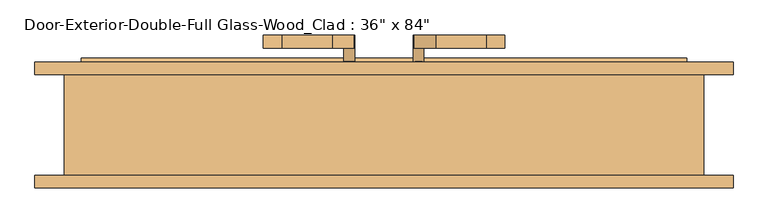
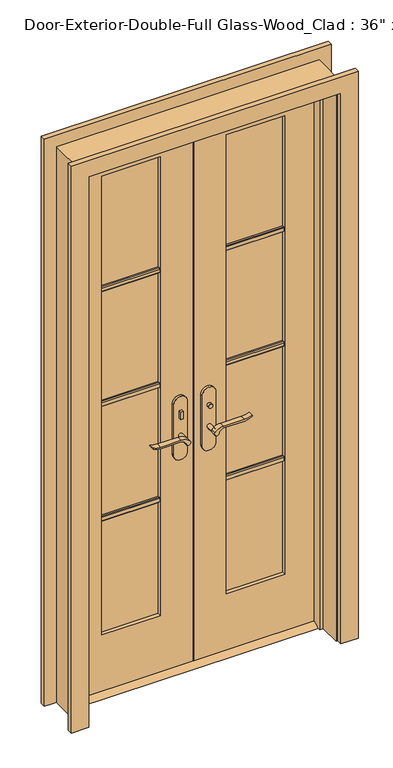
"""IFC4 building model written with IfcOpenShell, lengths in millimetres: door geometry."""

from ifc_helpers import new_model, si_unit, point, frame, frame_2d, origin, place, context, project, spatial, polyline, circle_curve, trimmed, segment, composite_curve, outline, extrude, faceted_brep, source, transform, mapped, element, save


def door_665efd91(model_context):
    return source(origin(), model_context, "Body", "SolidModel", [
        extrude(outline(polyline([(38.1, 12.7), (73.025, 12.7), (98.425, 0.0), (12.7, 0.0), (38.1, 12.7)])), frame((-457.2, 0.0, 0.0), z_axis=(1.0, 0.0, 0.0), x_axis=(0.0, 1.0, 0.0)), (0.0, 0.0, 1.0), 914.4),
        extrude(outline(polyline([(-47.4019111, 18.1), (-57.4019111, 18.1), (-57.4019111, 28.1), (-47.4019111, 28.1), (-47.4019111, 18.1)])), frame((0.0, 0.0, 981.9), z_axis=(0.0, 0.0, 1.0), x_axis=(1.0, 0.0, 0.0)), (0.0, 0.0, 1.0), 30.0),
        extrude(outline(composite_curve([segment(trimmed(circle_curve(frame_2d((996.9, -52.4019111)), 8.0), [point((996.9, -60.4019111))], [point((996.9, -44.4019111))], False, "CARTESIAN"), True, "CONTINUOUS"), segment(trimmed(circle_curve(frame_2d((996.9, -52.4019111)), 8.0), [point((996.9, -44.4019111))], [point((996.9, -60.4019111))], False, "CARTESIAN"), True, "CONTINUOUS")], self_intersect=False)), frame((0.0, 83.025, 0.0), z_axis=(0.0, 1.0, 0.0), x_axis=(0.0, 0.0, 1.0)), (0.0, 0.0, 1.0), 10.0),
        extrude(outline(composite_curve([segment(trimmed(circle_curve(frame_2d((897.1555521, -76.0694241)), 37.2832219), [point((919.0523287, -45.8937749))], [point((934.4, -77.7693445))], False, "CARTESIAN"), True, "CONTINUOUS"), segment(polyline([(934.4, -77.7693445), (934.4, -154.045502)]), True, "CONTINUOUS"), segment(trimmed(circle_curve(frame_2d((1017.6850638, -153.9791202)), 83.2850902), [point((934.4, -154.045502))], [point((939.4, -182.4019111))], True, "CARTESIAN"), True, "CONTINUOUS"), segment(polyline([(939.4, -182.4019111), (936.6135558, -182.4019111)]), True, "CONTINUOUS"), segment(trimmed(circle_curve(frame_2d((986.6709207, -150.4622499)), 59.3791355), [point((936.6135558, -182.4019111))], [point((927.4, -154.045502))], False, "CARTESIAN"), True, "CONTINUOUS"), segment(polyline([(927.4, -154.045502), (927.4, -77.7881013)]), True, "CONTINUOUS"), segment(trimmed(circle_curve(frame_2d((909.2738613, -77.7881013)), 18.1261387), [point((927.4, -77.7881013))], [point((914.4, -60.4019111))], True, "CARTESIAN"), True, "CONTINUOUS"), segment(trimmed(circle_curve(frame_2d((914.4, -52.4019111)), 8.0), [point((914.4, -60.4019111))], [point((919.0523287, -45.8937749))], False, "CARTESIAN"), True, "CONTINUOUS")], self_intersect=False)), frame((0.0, -21.9, 0.0), z_axis=(0.0, 1.0, 0.0), x_axis=(0.0, 0.0, 1.0)), (0.0, 0.0, 1.0), 20.0),
        extrude(outline(composite_curve([segment(trimmed(circle_curve(frame_2d((914.4, -52.4019111)), 8.0), [point((914.3999903, -60.4019111))], [point((919.0523287, -45.8937749))], False, "CARTESIAN"), True, "CONTINUOUS"), segment(trimmed(circle_curve(frame_2d((897.1555521, -76.0694241)), 37.2832219), [point((919.0523287, -45.8937749))], [point((934.4, -77.7693445))], False, "CARTESIAN"), True, "CONTINUOUS"), segment(polyline([(934.4, -77.7693445), (934.4, -154.045502)]), True, "CONTINUOUS"), segment(trimmed(circle_curve(frame_2d((1017.6850638, -153.9791202)), 83.2850902), [point((934.4, -154.045502))], [point((939.4, -182.4019111))], True, "CARTESIAN"), True, "CONTINUOUS"), segment(polyline([(939.4, -182.4019111), (936.6135558, -182.4019111)]), True, "CONTINUOUS"), segment(trimmed(circle_curve(frame_2d((986.6709207, -150.4622499)), 59.3791355), [point((936.6135558, -182.4019111))], [point((927.4, -154.045502))], False, "CARTESIAN"), True, "CONTINUOUS"), segment(polyline([(927.4, -154.045502), (927.4, -77.788099)]), True, "CONTINUOUS"), segment(trimmed(circle_curve(frame_2d((909.2738682, -77.788099)), 18.1261318), [point((927.4, -77.788099))], [point((914.3999903, -60.4019111))], True, "CARTESIAN"), True, "CONTINUOUS")], self_intersect=False)), frame((0.0, 113.025, 0.0), z_axis=(0.0, 1.0, 0.0), x_axis=(0.0, 0.0, 1.0)), (0.0, 0.0, 1.0), 20.0),
        extrude(outline(composite_curve([segment(trimmed(circle_curve(frame_2d((914.4, -52.4019111)), 8.0), [point((914.4, -60.4019111))], [point((914.4, -44.4019111))], False, "CARTESIAN"), True, "CONTINUOUS"), segment(trimmed(circle_curve(frame_2d((914.4, -52.4019111)), 8.0), [point((914.4, -44.4019111))], [point((914.4, -60.4019111))], False, "CARTESIAN"), True, "CONTINUOUS")], self_intersect=False)), frame((0.0, -1.9, 0.0), z_axis=(0.0, 1.0, 0.0), x_axis=(0.0, 0.0, 1.0)), (0.0, 0.0, 1.0), 30.0),
        extrude(outline(composite_curve([segment(trimmed(circle_curve(frame_2d((914.4, -52.4019111)), 8.0), [point((914.4, -60.4019111))], [point((914.4, -44.4019111))], False, "CARTESIAN"), True, "CONTINUOUS"), segment(trimmed(circle_curve(frame_2d((914.4, -52.4019111)), 8.0), [point((914.4, -44.4019111))], [point((914.4, -60.4019111))], False, "CARTESIAN"), True, "CONTINUOUS")], self_intersect=False)), frame((0.0, 83.025, 0.0), z_axis=(0.0, 1.0, 0.0), x_axis=(0.0, 0.0, 1.0)), (0.0, 0.0, 1.0), 30.0),
        extrude(outline(composite_curve([segment(polyline([(844.4, -27.4019111), (1039.4, -27.4019111)]), True, "CONTINUOUS"), segment(trimmed(circle_curve(frame_2d((1039.4, -52.4019111)), 25.0), [point((1039.4, -27.4019111))], [point((1039.4, -77.4019111))], False, "CARTESIAN"), True, "CONTINUOUS"), segment(polyline([(1039.4, -77.4019111), (844.4, -77.4019111)]), True, "CONTINUOUS"), segment(trimmed(circle_curve(frame_2d((844.4, -52.4019111)), 25.0), [point((844.4, -77.4019111))], [point((844.4, -27.4019111))], False, "CARTESIAN"), True, "CONTINUOUS")], self_intersect=False)), frame((0.0, 28.1, 0.0), z_axis=(0.0, 1.0, 0.0), x_axis=(0.0, 0.0, 1.0)), (0.0, 0.0, 1.0), 10.0),
        extrude(outline(composite_curve([segment(polyline([(844.4, -27.4019111), (1039.4, -27.4019111)]), True, "CONTINUOUS"), segment(trimmed(circle_curve(frame_2d((1039.4, -52.4019111)), 25.0), [point((1039.4, -27.4019111))], [point((1039.4, -77.4019111))], False, "CARTESIAN"), True, "CONTINUOUS"), segment(polyline([(1039.4, -77.4019111), (844.4, -77.4019111)]), True, "CONTINUOUS"), segment(trimmed(circle_curve(frame_2d((844.4, -52.4019111)), 25.0), [point((844.4, -77.4019111))], [point((844.4, -27.4019111))], False, "CARTESIAN"), True, "CONTINUOUS")], self_intersect=False)), frame((0.0, 73.025, 0.0), z_axis=(0.0, 1.0, 0.0), x_axis=(0.0, 0.0, 1.0)), (0.0, 0.0, 1.0), 10.0),
        extrude(outline(polyline([(47.3875, 93.025), (57.3875, 93.025), (57.3875, 83.025), (47.3875, 83.025), (47.3875, 93.025)])), frame((0.0, 0.0, 981.9), z_axis=(0.0, 0.0, 1.0), x_axis=(1.0, 0.0, 0.0)), (0.0, 0.0, 1.0), 30.0),
        extrude(outline(composite_curve([segment(trimmed(circle_curve(frame_2d((996.9, 52.3875)), 8.0), [point((996.9, 60.3875))], [point((996.9, 44.3875))], False, "CARTESIAN"), True, "CONTINUOUS"), segment(trimmed(circle_curve(frame_2d((996.9, 52.3875)), 8.0), [point((996.9, 44.3875))], [point((996.9, 60.3875))], False, "CARTESIAN"), True, "CONTINUOUS")], self_intersect=False)), frame((0.0, 18.1, 0.0), z_axis=(0.0, 1.0, 0.0), x_axis=(0.0, 0.0, 1.0)), (0.0, 0.0, 1.0), 10.0),
        extrude(outline(composite_curve([segment(trimmed(circle_curve(frame_2d((914.4, 52.3875)), 8.0), [point((919.0523287, 45.8793637))], [point((914.4, 60.3875))], False, "CARTESIAN"), True, "CONTINUOUS"), segment(trimmed(circle_curve(frame_2d((909.2738613, 77.7736901)), 18.1261387), [point((914.4, 60.3875))], [point((927.4, 77.7736901))], True, "CARTESIAN"), True, "CONTINUOUS"), segment(polyline([(927.4, 77.7736901), (927.4, 154.0310909)]), True, "CONTINUOUS"), segment(trimmed(circle_curve(frame_2d((986.6709207, 150.4478388)), 59.3791355), [point((927.4, 154.0310909))], [point((936.6135558, 182.3875))], False, "CARTESIAN"), True, "CONTINUOUS"), segment(polyline([(936.6135558, 182.3875), (939.4, 182.3875)]), True, "CONTINUOUS"), segment(trimmed(circle_curve(frame_2d((1017.6850638, 153.9647091)), 83.2850902), [point((939.4, 182.3875))], [point((934.4, 154.0310909))], True, "CARTESIAN"), True, "CONTINUOUS"), segment(polyline([(934.4, 154.0310909), (934.4, 77.7549333)]), True, "CONTINUOUS"), segment(trimmed(circle_curve(frame_2d((897.1555521, 76.0550129)), 37.2832219), [point((934.4, 77.7549333))], [point((919.0523287, 45.8793637))], False, "CARTESIAN"), True, "CONTINUOUS")], self_intersect=False)), frame((0.0, 113.025, 0.0), z_axis=(0.0, 1.0, 0.0), x_axis=(0.0, 0.0, 1.0)), (0.0, 0.0, 1.0), 20.0),
        extrude(outline(composite_curve([segment(trimmed(circle_curve(frame_2d((909.2738682, 77.7736878)), 18.1261318), [point((914.3999903, 60.3875))], [point((927.4, 77.7736878))], True, "CARTESIAN"), True, "CONTINUOUS"), segment(polyline([(927.4, 77.7736878), (927.4, 154.0310909)]), True, "CONTINUOUS"), segment(trimmed(circle_curve(frame_2d((986.6709207, 150.4478388)), 59.3791355), [point((927.4, 154.0310909))], [point((936.6135558, 182.3875))], False, "CARTESIAN"), True, "CONTINUOUS"), segment(polyline([(936.6135558, 182.3875), (939.4, 182.3875)]), True, "CONTINUOUS"), segment(trimmed(circle_curve(frame_2d((1017.6850638, 153.9647091)), 83.2850902), [point((939.4, 182.3875))], [point((934.4, 154.0310909))], True, "CARTESIAN"), True, "CONTINUOUS"), segment(polyline([(934.4, 154.0310909), (934.4, 77.7549333)]), True, "CONTINUOUS"), segment(trimmed(circle_curve(frame_2d((897.1555521, 76.0550129)), 37.2832219), [point((934.4, 77.7549333))], [point((919.0523287, 45.8793637))], False, "CARTESIAN"), True, "CONTINUOUS"), segment(trimmed(circle_curve(frame_2d((914.4, 52.3875)), 8.0), [point((919.0523287, 45.8793637))], [point((914.3999903, 60.3875))], False, "CARTESIAN"), True, "CONTINUOUS")], self_intersect=False)), frame((0.0, -21.9, 0.0), z_axis=(0.0, 1.0, 0.0), x_axis=(0.0, 0.0, 1.0)), (0.0, 0.0, 1.0), 20.0),
        extrude(outline(composite_curve([segment(trimmed(circle_curve(frame_2d((914.4, 52.3875)), 8.0), [point((914.4, 60.3875))], [point((914.4, 44.3875))], False, "CARTESIAN"), True, "CONTINUOUS"), segment(trimmed(circle_curve(frame_2d((914.4, 52.3875)), 8.0), [point((914.4, 44.3875))], [point((914.4, 60.3875))], False, "CARTESIAN"), True, "CONTINUOUS")], self_intersect=False)), frame((0.0, 83.025, 0.0), z_axis=(0.0, 1.0, 0.0), x_axis=(0.0, 0.0, 1.0)), (0.0, 0.0, 1.0), 30.0),
        extrude(outline(composite_curve([segment(trimmed(circle_curve(frame_2d((914.4, 52.3875)), 8.0), [point((914.4, 60.3875))], [point((914.4, 44.3875))], False, "CARTESIAN"), True, "CONTINUOUS"), segment(trimmed(circle_curve(frame_2d((914.4, 52.3875)), 8.0), [point((914.4, 44.3875))], [point((914.4, 60.3875))], False, "CARTESIAN"), True, "CONTINUOUS")], self_intersect=False)), frame((0.0, -1.9, 0.0), z_axis=(0.0, 1.0, 0.0), x_axis=(0.0, 0.0, 1.0)), (0.0, 0.0, 1.0), 30.0),
        extrude(outline(composite_curve([segment(trimmed(circle_curve(frame_2d((844.4, 52.3875)), 25.0), [point((844.4, 27.3875))], [point((844.4, 77.3875))], False, "CARTESIAN"), True, "CONTINUOUS"), segment(polyline([(844.4, 77.3875), (1039.4, 77.3875)]), True, "CONTINUOUS"), segment(trimmed(circle_curve(frame_2d((1039.4, 52.3875)), 25.0), [point((1039.4, 77.3875))], [point((1039.4, 27.3875))], False, "CARTESIAN"), True, "CONTINUOUS"), segment(polyline([(1039.4, 27.3875), (844.4, 27.3875)]), True, "CONTINUOUS")], self_intersect=False)), frame((0.0, 73.025, 0.0), z_axis=(0.0, 1.0, 0.0), x_axis=(0.0, 0.0, 1.0)), (0.0, 0.0, 1.0), 10.0),
        extrude(outline(composite_curve([segment(trimmed(circle_curve(frame_2d((844.4, 52.3875)), 25.0), [point((844.4, 27.3875))], [point((844.4, 77.3875))], False, "CARTESIAN"), True, "CONTINUOUS"), segment(polyline([(844.4, 77.3875), (1039.4, 77.3875)]), True, "CONTINUOUS"), segment(trimmed(circle_curve(frame_2d((1039.4, 52.3875)), 25.0), [point((1039.4, 77.3875))], [point((1039.4, 27.3875))], False, "CARTESIAN"), True, "CONTINUOUS"), segment(polyline([(1039.4, 27.3875), (844.4, 27.3875)]), True, "CONTINUOUS")], self_intersect=False)), frame((0.0, 28.1, 0.0), z_axis=(0.0, 1.0, 0.0), x_axis=(0.0, 0.0, 1.0)), (0.0, 0.0, 1.0), 10.0),
        extrude(outline(polyline([(52.07, 1578.371875), (52.07, 1559.321875), (45.72, 1559.321875), (42.545, 1562.496875), (42.545, 1575.196875), (45.72, 1578.371875), (52.07, 1578.371875)])), frame((120.65, 0.0, 0.0), z_axis=(1.0, 0.0, 0.0), x_axis=(0.0, 1.0, 0.0)), (0.0, 0.0, 1.0), 215.9),
        extrude(outline(polyline([(52.07, 1132.68125), (52.07, 1113.63125), (45.72, 1113.63125), (42.545, 1116.80625), (42.545, 1129.50625), (45.72, 1132.68125), (52.07, 1132.68125)])), frame((120.65, 0.0, 0.0), z_axis=(1.0, 0.0, 0.0), x_axis=(0.0, 1.0, 0.0)), (0.0, 0.0, 1.0), 215.9),
        extrude(outline(polyline([(52.07, 686.990625), (52.07, 667.940625), (45.72, 667.940625), (42.545, 671.115625), (42.545, 683.815625), (45.72, 686.990625), (52.07, 686.990625)])), frame((120.65, 0.0, 0.0), z_axis=(1.0, 0.0, 0.0), x_axis=(0.0, 1.0, 0.0)), (0.0, 0.0, 1.0), 215.9),
        extrude(outline(polyline([(59.055, 1578.371875), (65.405, 1578.371875), (68.58, 1575.196875), (68.58, 1562.496875), (65.405, 1559.321875), (59.055, 1559.321875), (59.055, 1578.371875)])), frame((-336.55, 0.0, 0.0), z_axis=(1.0, 0.0, 0.0), x_axis=(0.0, 1.0, 0.0)), (0.0, 0.0, 1.0), 215.9),
        extrude(outline(polyline([(59.055, 1132.68125), (65.405, 1132.68125), (68.58, 1129.50625), (68.58, 1116.80625), (65.405, 1113.63125), (59.055, 1113.63125), (59.055, 1132.68125)])), frame((-336.55, 0.0, 0.0), z_axis=(1.0, 0.0, 0.0), x_axis=(0.0, 1.0, 0.0)), (0.0, 0.0, 1.0), 215.9),
        extrude(outline(polyline([(59.055, 686.990625), (65.405, 686.990625), (68.58, 683.815625), (68.58, 671.115625), (65.405, 667.940625), (59.055, 667.940625), (59.055, 686.990625)])), frame((-336.55, 0.0, 0.0), z_axis=(1.0, 0.0, 0.0), x_axis=(0.0, 1.0, 0.0)), (0.0, 0.0, 1.0), 215.9),
        extrude(outline(polyline([(59.055, 1578.371875), (65.405, 1578.371875), (68.58, 1575.196875), (68.58, 1562.496875), (65.405, 1559.321875), (59.055, 1559.321875), (59.055, 1578.371875)])), frame((120.65, 0.0, 0.0), z_axis=(1.0, 0.0, 0.0), x_axis=(0.0, 1.0, 0.0)), (0.0, 0.0, 1.0), 215.9),
        extrude(outline(polyline([(59.055, 1132.68125), (65.405, 1132.68125), (68.58, 1129.50625), (68.58, 1116.80625), (65.405, 1113.63125), (59.055, 1113.63125), (59.055, 1132.68125)])), frame((120.65, 0.0, 0.0), z_axis=(1.0, 0.0, 0.0), x_axis=(0.0, 1.0, 0.0)), (0.0, 0.0, 1.0), 215.9),
        extrude(outline(polyline([(59.055, 686.990625), (65.405, 686.990625), (68.58, 683.815625), (68.58, 671.115625), (65.405, 667.940625), (59.055, 667.940625), (59.055, 686.990625)])), frame((120.65, 0.0, 0.0), z_axis=(1.0, 0.0, 0.0), x_axis=(0.0, 1.0, 0.0)), (0.0, 0.0, 1.0), 215.9),
        extrude(outline(polyline([(52.07, 1578.371875), (52.07, 1559.321875), (45.72, 1559.321875), (42.545, 1562.496875), (42.545, 1575.196875), (45.72, 1578.371875), (52.07, 1578.371875)])), frame((-336.55, 0.0, 0.0), z_axis=(1.0, 0.0, 0.0), x_axis=(0.0, 1.0, 0.0)), (0.0, 0.0, 1.0), 215.9),
        extrude(outline(polyline([(52.07, 1132.68125), (52.07, 1113.63125), (45.72, 1113.63125), (42.545, 1116.80625), (42.545, 1129.50625), (45.72, 1132.68125), (52.07, 1132.68125)])), frame((-336.55, 0.0, 0.0), z_axis=(1.0, 0.0, 0.0), x_axis=(0.0, 1.0, 0.0)), (0.0, 0.0, 1.0), 215.9),
        extrude(outline(polyline([(52.07, 686.990625), (52.07, 667.940625), (45.72, 667.940625), (42.545, 671.115625), (42.545, 683.815625), (45.72, 686.990625), (52.07, 686.990625)])), frame((-336.55, 0.0, 0.0), z_axis=(1.0, 0.0, 0.0), x_axis=(0.0, 1.0, 0.0)), (0.0, 0.0, 1.0), 215.9),
        extrude(outline(polyline([(0.0, 463.55), (0.0, 527.05), (2203.45, 527.05), (2203.45, -527.05), (0.0, -527.05), (0.0, -463.55), (2139.95, -463.55), (2139.95, 463.55), (0.0, 463.55)])), frame((0.0, 73.025, 0.0), z_axis=(0.0, 1.0, 0.0), x_axis=(0.0, 0.0, 1.0)), (0.0, 0.0, 1.0), 19.05),
        extrude(outline(polyline([(0.0, 463.55), (0.0, 527.05), (2203.45, 527.05), (2203.45, -527.05), (0.0, -527.05), (0.0, -463.55), (2139.95, -463.55), (2139.95, 463.55), (0.0, 463.55)])), frame((0.0, -98.425, 0.0), z_axis=(0.0, 1.0, 0.0), x_axis=(0.0, 0.0, 1.0)), (0.0, 0.0, 1.0), 19.05),
        extrude(outline(polyline([(12.7, 457.2), (2133.6, 457.2), (2133.6, 1.5875), (12.7, 1.5875), (12.7, 457.2)]), holes=[polyline([(2014.5375, 120.65), (2014.5375, 336.55), (231.775, 336.55), (231.775, 120.65), (2014.5375, 120.65)])]), frame((0.0, 38.1, 0.0), z_axis=(0.0, 1.0, 0.0), x_axis=(0.0, 0.0, 1.0)), (0.0, 0.0, 1.0), 34.925),
        extrude(outline(polyline([(2133.6, -457.2), (12.7, -457.2), (12.7, -1.6019111), (2133.6, -1.6019111), (2133.6, -457.2)]), holes=[polyline([(231.775, -336.55), (2014.5375, -336.55), (2014.5375, -120.65), (231.775, -120.65), (231.775, -336.55)])]), frame((0.0, 38.1, 0.0), z_axis=(0.0, 1.0, 0.0), x_axis=(0.0, 0.0, 1.0)), (0.0, 0.0, 1.0), 34.925),
        faceted_brep([(482.6, 73.025, 0.0), (482.6, -79.375, 0.0), (457.2, -79.375, 0.0), (457.2, 3.175, 0.0), (444.5, 3.175, 0.0), (444.5, 38.1, 0.0), (457.2, 38.1, 0.0), (457.2, 73.025, 0.0), (482.6, 73.025, 2159.0), (482.6, -79.375, 2159.0), (-482.6, -79.375, 2159.0), (-482.6, -79.375, 0.0), (-457.2, -79.375, 0.0), (-457.2, -79.375, 2133.6), (457.2, -79.375, 2133.6), (457.2, 3.175, 2133.6), (-457.2, 3.175, 2133.6), (-457.2, 3.175, 0.0), (-444.5, 3.175, 0.0), (-444.5, 3.175, 2120.9), (444.5, 3.175, 2120.9), (444.5, 38.1, 2120.9), (1.5875, 38.1, 2120.9), (-1.6019111, 38.1, 2120.9), (-444.5, 38.1, 2120.9), (-444.5, 38.1, 0.0), (-457.2, 38.1, 0.0), (-457.2, 38.1, 2133.6), (-1.6019111, 38.1, 2133.6), (1.5875, 38.1, 2133.6), (457.2, 38.1, 2133.6), (457.2, 73.025, 2133.6), (1.5875, 73.025, 2133.6), (-1.6019111, 73.025, 2133.6), (-457.2, 73.025, 2133.6), (-457.2, 73.025, 0.0), (-482.6, 73.025, 0.0), (-482.6, 73.025, 2159.0)], [[[0, 1, 2, 3, 4, 5, 6, 7]], [[1, 0, 8, 9]], [[2, 1, 9, 10, 11, 12, 13, 14]], [[3, 2, 14, 15]], [[4, 3, 15, 16, 17, 18, 19, 20]], [[5, 4, 20, 21]], [[6, 5, 21, 22, 23, 24, 25, 26, 27, 28, 29, 30]], [[7, 6, 30, 31]], [[0, 7, 31, 32, 33, 34, 35, 36, 37, 8]], [[9, 8, 37, 10]], [[14, 13, 16, 15]], [[20, 19, 24, 23, 22, 21]], [[31, 30, 29, 28, 27, 34, 33, 32]], [[12, 11, 36, 35, 26, 25, 18, 17]], [[11, 10, 37, 36]], [[13, 12, 17, 16]], [[19, 18, 25, 24]], [[27, 26, 35, 34]]]),
        extrude(outline(polyline([(336.55, 52.07), (120.65, 52.07), (120.65, 59.055), (336.55, 59.055), (336.55, 52.07)])), frame((0.0, 0.0, 231.775), z_axis=(0.0, 0.0, 1.0), x_axis=(1.0, 0.0, 0.0)), (0.0, 0.0, 1.0), 1782.7625),
        extrude(outline(polyline([(-120.65, 52.07), (-336.55, 52.07), (-336.55, 59.055), (-120.65, 59.055), (-120.65, 52.07)])), frame((0.0, 0.0, 231.775), z_axis=(0.0, 0.0, 1.0), x_axis=(1.0, 0.0, 0.0)), (0.0, 0.0, 1.0), 1782.7625),
    ])


if __name__ == "__main__":
    model = new_model("IFC4")
    model_context = context("Model", 3, world=origin())
    ifc_project = project(units=[si_unit("LENGTHUNIT", "METRE", prefix="MILLI")], contexts=[model_context])
    site = spatial("IfcSite", under=ifc_project)
    building = spatial("IfcBuilding", under=site)
    placement = place(None, origin())
    door_shape = door_665efd91(model_context)
    element("IfcDoor", 1, ObjectType="Door-Exterior-Double-Full Glass-Wood_Clad : 36\" x 84\"", at=placement, inside=building, context=model_context, shape_type="MappedRepresentation", body=[
        mapped(door_shape, transform((0.0, 0.0, 0.0), x_axis=(1.0, 0.0, 0.0), y_axis=(0.0, 1.0, 0.0), z_axis=(0.0, 0.0, 1.0))),
    ])
    save(model, "model.ifc")

# Revit data of these elements
# Type "Door-Exterior-Double-Full Glass-Wood_Clad : 36\" x 84\""
#   Type Mark = "10"
#   Assembly Code = "B2030100"
#   Analytic Construction = "French door, wood frame with double glass"
#   Top Rail = 0' - 4 11/16"
#   Threshold Offset [instance default] = 0' - 0 1/2"
#   Thickness = 0' - 1 3/8"
#   Thermal Resistance (R) = 1.9158 (h·ft²·°F)/BTU
#   Swing Angle [instance default] = 90.00°
#   Stiles = 0' - 4 3/4"
#   Rough Width = 3' - 2"
#   Rough Height = 7' - 1"
#   Panel Width = 1' - 6"
#   Door Offset [instance default] = 0' - 0"
#   Height = 7' - 0"
#   Width = 3' - 0"
#   Heat Transfer Coefficient (U) = 0.5220 BTU/(h·ft²·°F)
#   Bottom Rail = 0' - 9 1/8"
#   Exterior Trim [instance default] = yes
#   Threshold [instance default] = yes
#   Show Grill [instance default] = yes
#   Function = 1
#   Trim Material = Cherry
#   Threshold Material = Cherry
#   Panel Material = Cherry
#   Glazing = Glass
#   Frame Material = Cherry
#   Door Handle Material = Aluminum
#   Visual Light Transmittance = 0
#   Solar Heat Gain Coefficient = 0
#   Wall Closure = (empty or 0)
#   Construction Type = (empty or 0)
# Element 1 (IfcDoor, "Door-Exterior-Double-Full Glass-Wood_Clad : 36\" x 84\"")
#   Materials on its faces: "Cherry", "Aluminum", "Glass"
# Materials
#   "Cherry": class "Wood", colour RGB 226 177 128, transparency 0, Description = "Prunus Serotina", Cost = 0
#   "Glass": class "Glass", colour RGB 0 128 192, transparency 0.75, Description = "Soda Lime Glass", Cost = 0
#   "Aluminum": class "Metal", colour RGB 247 247 247, transparency 0, Description = "Aluminum 6061", Cost = 0
